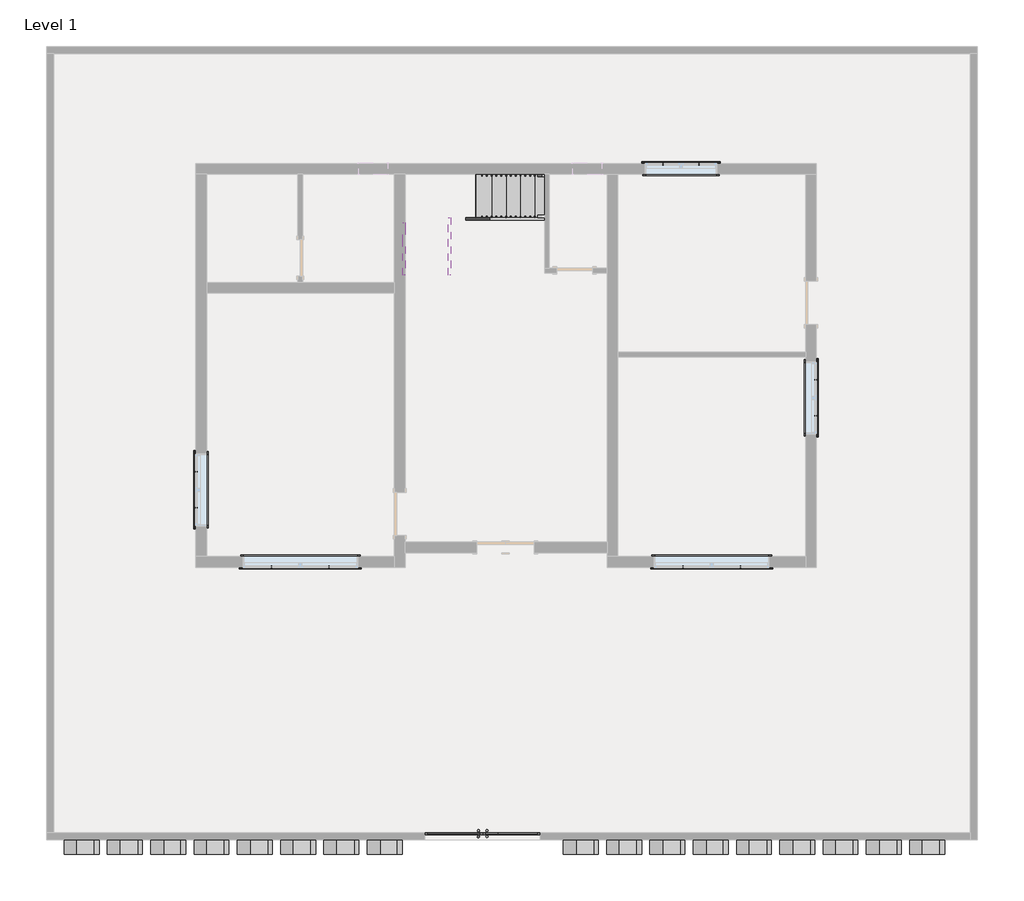
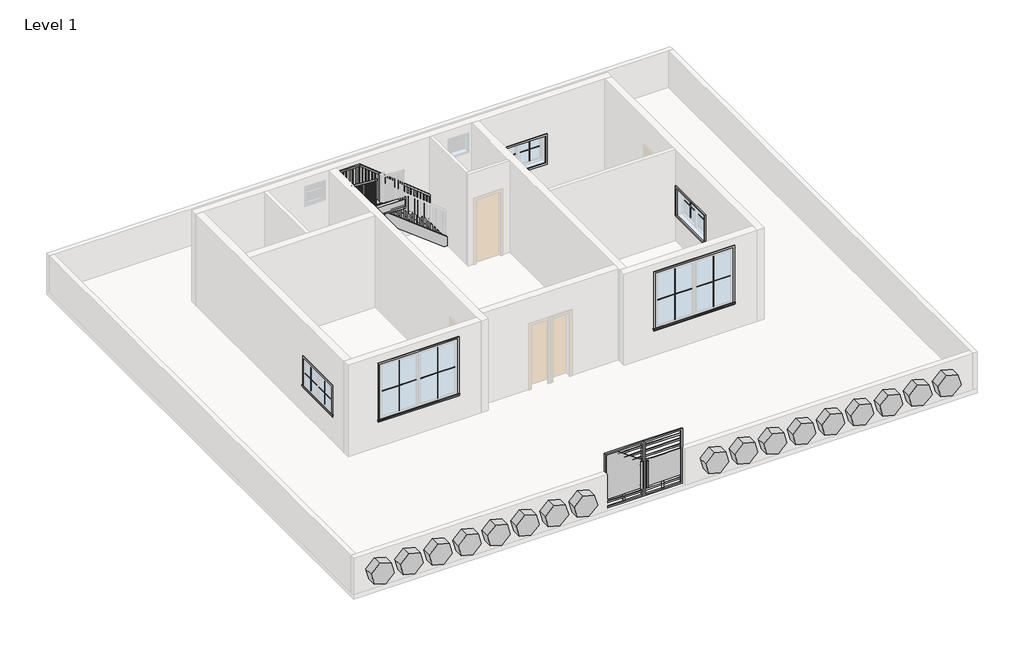
# One storey, part 2 of 2: 38 proxies, 4 members, 1 railing, 1 stair flight.
"""IFC4 building model written with IfcOpenShell, lengths in millimetres."""

from ifc_helpers import new_model, si_unit, frame, origin, place, context, project, spatial, polyline, outline, extrude, faceted_brep, transform, mapped, element, save
from components import generic_models_113f6068, generic_models_1_generic_models_1_e32cbfde, generic_models_10_generic_models_1_db47fcfa, generic_models_11_generic_models_1_4c9ee5e0, generic_models_12_generic_models_1_cd0b2d88, generic_models_13_generic_models_1_344792cf, generic_models_14_generic_models_1_1a1bfa67, generic_models_15_generic_models_1_a1369ee7, generic_models_16_generic_models_1_a0735545, generic_models_17_generic_models_1_fcac293f, generic_models_2_generic_models_1_372cb617, generic_models_3_generic_models_1_c8895c90, generic_models_4_generic_models_1_1de10410, generic_models_5_generic_models_1_6e22be36, generic_models_6_generic_models_1_19455b19, generic_models_7_generic_models_1_35c4f0a6, generic_models_8_generic_models_1_b8e4b7b0, generic_models_9_generic_models_1_cc0d601c, muntin_pattern_2x2_muntin_pattern_2x2_9352d081, muntin_pattern_2x2_muntin_pattern_2x2_5c2cbe28, muntin_pattern_2x2_muntin_pattern_2x2_bb8d4d84, muntin_pattern_2x2_muntin_pattern_2x2_d03a1f3c, trim_window_exterior_flat_with_sill_979bde60, trim_window_exterior_flat_with_sill_359ed2ce, trim_window_interior_flat_picture_frame_7883d11b, trim_window_interior_flat_picture_frame_939a8053, stair_flight_e32d701a

model = new_model("IFC4")

# Units and contexts
model_context = context("Model", 3, world=origin())
ifc_project = project(units=[si_unit("LENGTHUNIT", "METRE", prefix="MILLI")], contexts=[model_context])

# Site, building, storey
site = spatial("IfcSite", under=ifc_project)
building = spatial("IfcBuilding", under=site)
storey = spatial("IfcBuildingStorey", under=building, Name="Level 1", Elevation=0.0)

# Proxies
placement = place(None, origin())
generic_models_shape = generic_models_113f6068(model_context)
element("IfcBuildingElementProxy", 1, Name="Generic Models", at=placement, inside=storey, context=model_context, shape_type="MappedRepresentation", body=[
    mapped(generic_models_shape, transform((-1750.5415084, -8629.4225464, 0.0), x_axis=(1.0, 0.0, 0.0), y_axis=(0.0, 1.0, 0.0), z_axis=(0.0, 0.0, 1.0))),
])
generic_models_1_generic_models_1_shape = generic_models_1_generic_models_1_e32cbfde(model_context)
element("IfcBuildingElementProxy", 2, Name="Generic Models 1 : Generic Models 1", ObjectType="Generic Models 1 : Generic Models 1", at=placement, inside=storey, context=model_context, shape_type="MappedRepresentation", body=[
    mapped(generic_models_1_generic_models_1_shape, transform((0.0, 0.0, 0.0), x_axis=(1.0, 0.0, 0.0), y_axis=(0.0, 1.0, 0.0), z_axis=(0.0, 0.0, 1.0))),
])
generic_models_10_generic_models_1_shape = generic_models_10_generic_models_1_db47fcfa(model_context)
element("IfcBuildingElementProxy", 3, Name="Generic Models 10 : Generic Models 1", ObjectType="Generic Models 10 : Generic Models 1", at=placement, inside=storey, context=model_context, shape_type="MappedRepresentation", body=[
    mapped(generic_models_10_generic_models_1_shape, transform((0.0, 0.0, 0.0), x_axis=(1.0, 0.0, 0.0), y_axis=(0.0, 1.0, 0.0), z_axis=(0.0, 0.0, 1.0))),
])
generic_models_11_generic_models_1_shape = generic_models_11_generic_models_1_4c9ee5e0(model_context)
element("IfcBuildingElementProxy", 4, Name="Generic Models 11 : Generic Models 1", ObjectType="Generic Models 11 : Generic Models 1", at=placement, inside=storey, context=model_context, shape_type="MappedRepresentation", body=[
    mapped(generic_models_11_generic_models_1_shape, transform((0.0, 0.0, 0.0), x_axis=(1.0, 0.0, 0.0), y_axis=(0.0, 1.0, 0.0), z_axis=(0.0, 0.0, 1.0))),
])
generic_models_12_generic_models_1_shape = generic_models_12_generic_models_1_cd0b2d88(model_context)
element("IfcBuildingElementProxy", 5, Name="Generic Models 12 : Generic Models 1", ObjectType="Generic Models 12 : Generic Models 1", at=placement, inside=storey, context=model_context, shape_type="MappedRepresentation", body=[
    mapped(generic_models_12_generic_models_1_shape, transform((0.0, 0.0, 0.0), x_axis=(1.0, 0.0, 0.0), y_axis=(0.0, 1.0, 0.0), z_axis=(0.0, 0.0, 1.0))),
])
generic_models_13_generic_models_1_shape = generic_models_13_generic_models_1_344792cf(model_context)
element("IfcBuildingElementProxy", 6, Name="Generic Models 13 : Generic Models 1", ObjectType="Generic Models 13 : Generic Models 1", at=placement, inside=storey, context=model_context, shape_type="MappedRepresentation", body=[
    mapped(generic_models_13_generic_models_1_shape, transform((0.0, 0.0, 0.0), x_axis=(1.0, 0.0, 0.0), y_axis=(0.0, 1.0, 0.0), z_axis=(0.0, 0.0, 1.0))),
])
generic_models_14_generic_models_1_shape = generic_models_14_generic_models_1_1a1bfa67(model_context)
element("IfcBuildingElementProxy", 7, Name="Generic Models 14 : Generic Models 1", ObjectType="Generic Models 14 : Generic Models 1", at=placement, inside=storey, context=model_context, shape_type="MappedRepresentation", body=[
    mapped(generic_models_14_generic_models_1_shape, transform((0.0, 0.0, 0.0), x_axis=(1.0, 0.0, 0.0), y_axis=(0.0, 1.0, 0.0), z_axis=(0.0, 0.0, 1.0))),
])
generic_models_15_generic_models_1_shape = generic_models_15_generic_models_1_a1369ee7(model_context)
element("IfcBuildingElementProxy", 8, Name="Generic Models 15 : Generic Models 1", ObjectType="Generic Models 15 : Generic Models 1", at=placement, inside=storey, context=model_context, shape_type="MappedRepresentation", body=[
    mapped(generic_models_15_generic_models_1_shape, transform((0.0, 0.0, 0.0), x_axis=(1.0, 0.0, 0.0), y_axis=(0.0, 1.0, 0.0), z_axis=(0.0, 0.0, 1.0))),
])
generic_models_16_generic_models_1_shape = generic_models_16_generic_models_1_a0735545(model_context)
element("IfcBuildingElementProxy", 9, Name="Generic Models 16 : Generic Models 1", ObjectType="Generic Models 16 : Generic Models 1", at=placement, inside=storey, context=model_context, shape_type="MappedRepresentation", body=[
    mapped(generic_models_16_generic_models_1_shape, transform((0.0, 0.0, 0.0), x_axis=(1.0, 0.0, 0.0), y_axis=(0.0, 1.0, 0.0), z_axis=(0.0, 0.0, 1.0))),
])
generic_models_17_generic_models_1_shape = generic_models_17_generic_models_1_fcac293f(model_context)
element("IfcBuildingElementProxy", 10, Name="Generic Models 17 : Generic Models 1", ObjectType="Generic Models 17 : Generic Models 1", at=placement, inside=storey, context=model_context, shape_type="MappedRepresentation", body=[
    mapped(generic_models_17_generic_models_1_shape, transform((0.0, 0.0, 0.0), x_axis=(1.0, 0.0, 0.0), y_axis=(0.0, 1.0, 0.0), z_axis=(0.0, 0.0, 1.0))),
])
generic_models_2_generic_models_1_shape = generic_models_2_generic_models_1_372cb617(model_context)
element("IfcBuildingElementProxy", 11, Name="Generic Models 2 : Generic Models 1", ObjectType="Generic Models 2 : Generic Models 1", at=placement, inside=storey, context=model_context, shape_type="MappedRepresentation", body=[
    mapped(generic_models_2_generic_models_1_shape, transform((0.0, 0.0, 0.0), x_axis=(1.0, 0.0, 0.0), y_axis=(0.0, 1.0, 0.0), z_axis=(0.0, 0.0, 1.0))),
])
generic_models_3_generic_models_1_shape = generic_models_3_generic_models_1_c8895c90(model_context)
element("IfcBuildingElementProxy", 12, Name="Generic Models 3 : Generic Models 1", ObjectType="Generic Models 3 : Generic Models 1", at=placement, inside=storey, context=model_context, shape_type="MappedRepresentation", body=[
    mapped(generic_models_3_generic_models_1_shape, transform((0.0, 0.0, 0.0), x_axis=(1.0, 0.0, 0.0), y_axis=(0.0, 1.0, 0.0), z_axis=(0.0, 0.0, 1.0))),
])
generic_models_4_generic_models_1_shape = generic_models_4_generic_models_1_1de10410(model_context)
element("IfcBuildingElementProxy", 13, Name="Generic Models 4 : Generic Models 1", ObjectType="Generic Models 4 : Generic Models 1", at=placement, inside=storey, context=model_context, shape_type="MappedRepresentation", body=[
    mapped(generic_models_4_generic_models_1_shape, transform((0.0, 0.0, 0.0), x_axis=(1.0, 0.0, 0.0), y_axis=(0.0, 1.0, 0.0), z_axis=(0.0, 0.0, 1.0))),
])
generic_models_5_generic_models_1_shape = generic_models_5_generic_models_1_6e22be36(model_context)
element("IfcBuildingElementProxy", 14, Name="Generic Models 5 : Generic Models 1", ObjectType="Generic Models 5 : Generic Models 1", at=placement, inside=storey, context=model_context, shape_type="MappedRepresentation", body=[
    mapped(generic_models_5_generic_models_1_shape, transform((0.0, 0.0, 0.0), x_axis=(1.0, 0.0, 0.0), y_axis=(0.0, 1.0, 0.0), z_axis=(0.0, 0.0, 1.0))),
])
generic_models_6_generic_models_1_shape = generic_models_6_generic_models_1_19455b19(model_context)
element("IfcBuildingElementProxy", 15, Name="Generic Models 6 : Generic Models 1", ObjectType="Generic Models 6 : Generic Models 1", at=placement, inside=storey, context=model_context, shape_type="MappedRepresentation", body=[
    mapped(generic_models_6_generic_models_1_shape, transform((0.0, 0.0, 0.0), x_axis=(1.0, 0.0, 0.0), y_axis=(0.0, 1.0, 0.0), z_axis=(0.0, 0.0, 1.0))),
])
generic_models_7_generic_models_1_shape = generic_models_7_generic_models_1_35c4f0a6(model_context)
element("IfcBuildingElementProxy", 16, Name="Generic Models 7 : Generic Models 1", ObjectType="Generic Models 7 : Generic Models 1", at=placement, inside=storey, context=model_context, shape_type="MappedRepresentation", body=[
    mapped(generic_models_7_generic_models_1_shape, transform((0.0, 0.0, 0.0), x_axis=(1.0, 0.0, 0.0), y_axis=(0.0, 1.0, 0.0), z_axis=(0.0, 0.0, 1.0))),
])
generic_models_8_generic_models_1_shape = generic_models_8_generic_models_1_b8e4b7b0(model_context)
element("IfcBuildingElementProxy", 17, Name="Generic Models 8 : Generic Models 1", ObjectType="Generic Models 8 : Generic Models 1", at=placement, inside=storey, context=model_context, shape_type="MappedRepresentation", body=[
    mapped(generic_models_8_generic_models_1_shape, transform((0.0, 0.0, 0.0), x_axis=(1.0, 0.0, 0.0), y_axis=(0.0, 1.0, 0.0), z_axis=(0.0, 0.0, 1.0))),
])
generic_models_9_generic_models_1_shape = generic_models_9_generic_models_1_cc0d601c(model_context)
element("IfcBuildingElementProxy", 18, Name="Generic Models 9 : Generic Models 1", ObjectType="Generic Models 9 : Generic Models 1", at=placement, inside=storey, context=model_context, shape_type="MappedRepresentation", body=[
    mapped(generic_models_9_generic_models_1_shape, transform((0.0, 0.0, 0.0), x_axis=(1.0, 0.0, 0.0), y_axis=(0.0, 1.0, 0.0), z_axis=(0.0, 0.0, 1.0))),
])
muntin_pattern_2x2_muntin_pattern_2x2_shape = muntin_pattern_2x2_muntin_pattern_2x2_9352d081(model_context)
element("IfcBuildingElementProxy", 19, Name="Muntin Pattern_2x2 : Muntin Pattern_2x2", ObjectType="Muntin Pattern_2x2 : Muntin Pattern_2x2", at=placement, inside=storey, context=model_context, shape_type="MappedRepresentation", body=[
    mapped(muntin_pattern_2x2_muntin_pattern_2x2_shape, transform((-7798.9165084, -1764.5743005, 984.25), x_axis=(0.0, 1.0, 0.0), y_axis=(-1.0, 0.0, 0.0), z_axis=(0.0, 0.0, 1.0))),
])
element("IfcBuildingElementProxy", 20, Name="Muntin Pattern_2x2 : Muntin Pattern_2x2", ObjectType="Muntin Pattern_2x2 : Muntin Pattern_2x2", at=placement, inside=storey, context=model_context, shape_type="MappedRepresentation", body=[
    mapped(muntin_pattern_2x2_muntin_pattern_2x2_shape, transform((5288.4334916, 937.3506995, 984.25), x_axis=(0.0, -1.0, 0.0), y_axis=(1.0, 0.0, 0.0), z_axis=(0.0, 0.0, 1.0))),
])
element("IfcBuildingElementProxy", 21, Name="Muntin Pattern_2x2 : Muntin Pattern_2x2", ObjectType="Muntin Pattern_2x2 : Muntin Pattern_2x2", at=placement, inside=storey, context=model_context, shape_type="MappedRepresentation", body=[
    mapped(muntin_pattern_2x2_muntin_pattern_2x2_shape, transform((2061.0459916, 5501.4131995, 984.25), x_axis=(1.0, 0.0, 0.0), y_axis=(0.0, 1.0, 0.0), z_axis=(0.0, 0.0, 1.0))),
])
muntin_pattern_2x2_muntin_pattern_2x2_2_shape = muntin_pattern_2x2_muntin_pattern_2x2_5c2cbe28(model_context)
element("IfcBuildingElementProxy", 22, Name="Muntin Pattern_2x2 : Muntin Pattern_2x2", ObjectType="Muntin Pattern_2x2 : Muntin Pattern_2x2", at=placement, inside=storey, context=model_context, shape_type="MappedRepresentation", body=[
    mapped(muntin_pattern_2x2_muntin_pattern_2x2_2_shape, transform((-7798.9165084, -1005.7493005, 984.25), x_axis=(0.0, -1.0, 0.0), y_axis=(1.0, 0.0, 0.0), z_axis=(0.0, 0.0, 1.0))),
])
element("IfcBuildingElementProxy", 23, Name="Muntin Pattern_2x2 : Muntin Pattern_2x2", ObjectType="Muntin Pattern_2x2 : Muntin Pattern_2x2", at=placement, inside=storey, context=model_context, shape_type="MappedRepresentation", body=[
    mapped(muntin_pattern_2x2_muntin_pattern_2x2_2_shape, transform((5288.4334916, 178.5256995, 984.25), x_axis=(0.0, 1.0, 0.0), y_axis=(-1.0, 0.0, 0.0), z_axis=(0.0, 0.0, 1.0))),
])
element("IfcBuildingElementProxy", 24, Name="Muntin Pattern_2x2 : Muntin Pattern_2x2", ObjectType="Muntin Pattern_2x2 : Muntin Pattern_2x2", at=placement, inside=storey, context=model_context, shape_type="MappedRepresentation", body=[
    mapped(muntin_pattern_2x2_muntin_pattern_2x2_2_shape, transform((2819.8709916, 5501.4131995, 984.25), x_axis=(-1.0, 0.0, 0.0), y_axis=(0.0, -1.0, 0.0), z_axis=(0.0, 0.0, 1.0))),
])
muntin_pattern_2x2_muntin_pattern_2x2_3_shape = muntin_pattern_2x2_muntin_pattern_2x2_bb8d4d84(model_context)
element("IfcBuildingElementProxy", 25, Name="Muntin Pattern_2x2 : Muntin Pattern_2x2", ObjectType="Muntin Pattern_2x2 : Muntin Pattern_2x2", at=placement, inside=storey, context=model_context, shape_type="MappedRepresentation", body=[
    mapped(muntin_pattern_2x2_muntin_pattern_2x2_3_shape, transform((-4990.6290084, -3013.9368005, 984.25), x_axis=(-1.0, 0.0, 0.0), y_axis=(0.0, -1.0, 0.0), z_axis=(0.0, 0.0, 1.0))),
])
element("IfcBuildingElementProxy", 26, Name="Muntin Pattern_2x2 : Muntin Pattern_2x2", ObjectType="Muntin Pattern_2x2 : Muntin Pattern_2x2", at=placement, inside=storey, context=model_context, shape_type="MappedRepresentation", body=[
    mapped(muntin_pattern_2x2_muntin_pattern_2x2_3_shape, transform((3696.1709916, -3013.9368005, 984.25), x_axis=(-1.0, 0.0, 0.0), y_axis=(0.0, -1.0, 0.0), z_axis=(0.0, 0.0, 1.0))),
])
muntin_pattern_2x2_muntin_pattern_2x2_4_shape = muntin_pattern_2x2_muntin_pattern_2x2_d03a1f3c(model_context)
element("IfcBuildingElementProxy", 27, Name="Muntin Pattern_2x2 : Muntin Pattern_2x2", ObjectType="Muntin Pattern_2x2 : Muntin Pattern_2x2", at=placement, inside=storey, context=model_context, shape_type="MappedRepresentation", body=[
    mapped(muntin_pattern_2x2_muntin_pattern_2x2_4_shape, transform((-6206.6540084, -3013.9368005, 984.25), x_axis=(1.0, 0.0, 0.0), y_axis=(0.0, 1.0, 0.0), z_axis=(0.0, 0.0, 1.0))),
])
element("IfcBuildingElementProxy", 28, Name="Muntin Pattern_2x2 : Muntin Pattern_2x2", ObjectType="Muntin Pattern_2x2 : Muntin Pattern_2x2", at=placement, inside=storey, context=model_context, shape_type="MappedRepresentation", body=[
    mapped(muntin_pattern_2x2_muntin_pattern_2x2_4_shape, transform((2480.1459916, -3013.9368005, 984.25), x_axis=(1.0, 0.0, 0.0), y_axis=(0.0, 1.0, 0.0), z_axis=(0.0, 0.0, 1.0))),
])
trim_window_exterior_flat_with_sill_shape = trim_window_exterior_flat_with_sill_979bde60(model_context)
element("IfcBuildingElementProxy", 29, Name="Trim-Window-Exterior-Flat : with Sill", ObjectType="Trim-Window-Exterior-Flat : with Sill", at=placement, inside=storey, context=model_context, shape_type="MappedRepresentation", body=[
    mapped(trim_window_exterior_flat_with_sill_shape, transform((-7808.4415084, -1385.1618005, 1828.8), x_axis=(0.0, -1.0, 0.0), y_axis=(0.0, 0.0, 1.0), z_axis=(-1.0, 0.0, 0.0))),
])
element("IfcBuildingElementProxy", 30, Name="Trim-Window-Exterior-Flat : with Sill", ObjectType="Trim-Window-Exterior-Flat : with Sill", at=placement, inside=storey, context=model_context, shape_type="MappedRepresentation", body=[
    mapped(trim_window_exterior_flat_with_sill_shape, transform((5297.9584916, 557.9381995, 1828.8), x_axis=(0.0, 1.0, 0.0), y_axis=(0.0, 0.0, 1.0), z_axis=(1.0, 0.0, 0.0))),
])
element("IfcBuildingElementProxy", 31, Name="Trim-Window-Exterior-Flat : with Sill", ObjectType="Trim-Window-Exterior-Flat : with Sill", at=placement, inside=storey, context=model_context, shape_type="MappedRepresentation", body=[
    mapped(trim_window_exterior_flat_with_sill_shape, transform((2440.4584916, 5510.9381995, 1828.8), x_axis=(-1.0, 0.0, 0.0), y_axis=(0.0, 0.0, 1.0), z_axis=(0.0, 1.0, 0.0))),
])
trim_window_exterior_flat_with_sill_2_shape = trim_window_exterior_flat_with_sill_359ed2ce(model_context)
element("IfcBuildingElementProxy", 32, Name="Trim-Window-Exterior-Flat : with Sill", ObjectType="Trim-Window-Exterior-Flat : with Sill", at=placement, inside=storey, context=model_context, shape_type="MappedRepresentation", body=[
    mapped(trim_window_exterior_flat_with_sill_2_shape, transform((-5598.6415084, -3023.4618005, 2743.2), x_axis=(1.0, 0.0, 0.0), y_axis=(0.0, 0.0, 1.0), z_axis=(0.0, -1.0, 0.0))),
])
element("IfcBuildingElementProxy", 33, Name="Trim-Window-Exterior-Flat : with Sill", ObjectType="Trim-Window-Exterior-Flat : with Sill", at=placement, inside=storey, context=model_context, shape_type="MappedRepresentation", body=[
    mapped(trim_window_exterior_flat_with_sill_2_shape, transform((3088.1584916, -3023.4618005, 2743.2), x_axis=(1.0, 0.0, 0.0), y_axis=(0.0, 0.0, 1.0), z_axis=(0.0, -1.0, 0.0))),
])
trim_window_interior_flat_picture_frame_shape = trim_window_interior_flat_picture_frame_7883d11b(model_context)
element("IfcBuildingElementProxy", 34, Name="Trim-Window-Interior-Flat : Picture Frame", ObjectType="Trim-Window-Interior-Flat : Picture Frame", at=placement, inside=storey, context=model_context, shape_type="MappedRepresentation", body=[
    mapped(trim_window_interior_flat_picture_frame_shape, transform((-7579.8415084, -1385.1618005, 1828.8), x_axis=(0.0, 1.0, 0.0), y_axis=(0.0, 0.0, 1.0), z_axis=(1.0, 0.0, 0.0))),
])
element("IfcBuildingElementProxy", 35, Name="Trim-Window-Interior-Flat : Picture Frame", ObjectType="Trim-Window-Interior-Flat : Picture Frame", at=placement, inside=storey, context=model_context, shape_type="MappedRepresentation", body=[
    mapped(trim_window_interior_flat_picture_frame_shape, transform((5069.3584916, 557.9381995, 1828.8), x_axis=(0.0, -1.0, 0.0), y_axis=(0.0, 0.0, 1.0), z_axis=(-1.0, 0.0, 0.0))),
])
element("IfcBuildingElementProxy", 36, Name="Trim-Window-Interior-Flat : Picture Frame", ObjectType="Trim-Window-Interior-Flat : Picture Frame", at=placement, inside=storey, context=model_context, shape_type="MappedRepresentation", body=[
    mapped(trim_window_interior_flat_picture_frame_shape, transform((2440.4584916, 5282.3381995, 1828.8), x_axis=(1.0, 0.0, 0.0), y_axis=(0.0, 0.0, 1.0), z_axis=(0.0, -1.0, 0.0))),
])
trim_window_interior_flat_picture_frame_2_shape = trim_window_interior_flat_picture_frame_939a8053(model_context)
element("IfcBuildingElementProxy", 37, Name="Trim-Window-Interior-Flat : Picture Frame", ObjectType="Trim-Window-Interior-Flat : Picture Frame", at=placement, inside=storey, context=model_context, shape_type="MappedRepresentation", body=[
    mapped(trim_window_interior_flat_picture_frame_2_shape, transform((-5598.6415084, -2794.8618005, 2743.2), x_axis=(-1.0, 0.0, 0.0), y_axis=(0.0, 0.0, 1.0), z_axis=(0.0, 1.0, 0.0))),
])
element("IfcBuildingElementProxy", 38, Name="Trim-Window-Interior-Flat : Picture Frame", ObjectType="Trim-Window-Interior-Flat : Picture Frame", at=placement, inside=storey, context=model_context, shape_type="MappedRepresentation", body=[
    mapped(trim_window_interior_flat_picture_frame_2_shape, transform((3088.1584916, -2794.8618005, 2743.2), x_axis=(-1.0, 0.0, 0.0), y_axis=(0.0, 0.0, 1.0), z_axis=(0.0, 1.0, 0.0))),
])

# Members
element("IfcMember", 39, ObjectType="Stringer - 2\" Width", at=placement, inside=storey, context=model_context, shape_type="SweptSolid", body=[
    extrude(outline(polyline([(0.0, -442.4415084), (307.3626352, -442.4415084), (1831.3626352, -2423.6415084), (1446.8171203, -2423.6415084), (0.0, -542.779252), (0.0, -442.4415084)])), frame((0.0, 4317.5146777, 0.0), z_axis=(0.0, 1.0, 0.0), x_axis=(0.0, 0.0, 1.0)), (0.0, 0.0, 1.0), 50.8),
])
element("IfcMember", 40, ObjectType="Stringer - 2\" Width", at=placement, inside=storey, context=model_context, shape_type="SweptSolid", body=[
    extrude(outline(polyline([(4368.3146777, 2104.8645881), (4368.3146777, 1720.3778824), (3148.7383287, 2658.1275497), (3148.7383287, 3042.6142554), (4368.3146777, 2104.8645881)])), frame((-2474.4415084, 0.0, 0.0), z_axis=(1.0, 0.0, 0.0), x_axis=(0.0, 1.0, 0.0)), (0.0, 0.0, 1.0), 50.8),
])
element("IfcMember", 41, ObjectType="Stringer - 2\" Width", at=placement, inside=storey, context=model_context, shape_type="SweptSolid", body=[
    extrude(outline(polyline([(0.0, -442.4415084), (307.3626352, -442.4415084), (1402.0588522, -1865.5465904), (1402.0588522, -2365.4557598), (0.0, -542.779252), (0.0, -442.4415084)])), frame((0.0, 5282.3381995, 0.0), z_axis=(0.0, 1.0, 0.0), x_axis=(0.0, 0.0, 1.0)), (0.0, 0.0, 1.0), 50.8),
])
element("IfcMember", 42, ObjectType="Stringer - 2\" Width", at=placement, inside=storey, context=model_context, shape_type="SweptSolid", body=[
    extrude(outline(polyline([(3758.4927637, 2189.2786588), (3148.7383287, 2658.1275497), (3148.7383287, 3042.6142554), (4258.5312166, 2189.2786588), (3758.4927637, 2189.2786588)])), frame((-3439.6415084, 0.0, 0.0), z_axis=(1.0, 0.0, 0.0), x_axis=(0.0, 1.0, 0.0)), (0.0, 0.0, 1.0), 50.8),
])

# Railing
element("IfcRailing", 43, ObjectType="Handrail - Rectangular", at=placement, inside=storey, context=model_context, shape_type="SolidModel", body=[
    faceted_brep([(-442.4415084, 5231.5381995, 1148.8615385), (-442.4415084, 5231.5381995, 1083.5609717), (-442.4415084, 5282.3381995, 1083.5609717), (-442.4415084, 5282.3381995, 1148.8615385), (-2641.0608886, 5231.5381995, 2924.6694994), (-2659.0139713, 5231.5381995, 2873.8694994), (-2659.0139713, 5282.3381995, 2873.8694994), (-2641.0608886, 5282.3381995, 2924.6694994), (-3338.0415084, 5231.5381995, 2924.6694994), (-3338.0415084, 5231.5381995, 2873.8694994), (-3388.8415084, 5282.3381995, 2873.8694994), (-3388.8415084, 5282.3381995, 2924.6694994), (-3338.0415084, 4498.2044111, 2924.6694994), (-3338.0415084, 4480.9304428, 2873.8694994), (-3388.8415084, 4480.9304428, 2873.8694994), (-3388.8415084, 4498.2044111, 2924.6694994), (-3338.0415084, 3148.7383287, 3962.4), (-3388.8415084, 3148.7383287, 3962.4), (-3388.8415084, 3148.7383287, 3898.3164325), (-3338.0415084, 3148.7383287, 3898.3164325)], [[[0, 1, 2, 3]], [[1, 0, 4, 5]], [[2, 1, 5, 6]], [[3, 2, 6, 7]], [[0, 3, 7, 4]], [[5, 4, 8, 9]], [[6, 5, 9, 10]], [[7, 6, 10, 11]], [[4, 7, 11, 8]], [[9, 8, 12, 13]], [[10, 9, 13, 14]], [[11, 10, 14, 15]], [[8, 11, 15, 12]], [[16, 17, 18, 19]], [[13, 12, 16, 19]], [[14, 13, 19, 18]], [[15, 14, 18, 17]], [[12, 15, 17, 16]]]),
    extrude(outline(polyline([(3215.4131995, 3847.1162499), (3234.4631995, 3832.4669257), (3234.4631995, 2813.5384615), (3215.4131995, 2813.5384615), (3215.4131995, 3847.1162499)])), frame((-3372.9665084, 0.0, 0.0), z_axis=(1.0, 0.0, 0.0), x_axis=(0.0, 1.0, 0.0)), (0.0, 0.0, 1.0), 19.05),
    extrude(outline(polyline([(3317.0131995, 3768.9141687), (3336.0631995, 3754.2648446), (3336.0631995, 2813.5384615), (3317.0131995, 2813.5384615), (3317.0131995, 3768.9141687)])), frame((-3372.9665084, 0.0, 0.0), z_axis=(1.0, 0.0, 0.0), x_axis=(0.0, 1.0, 0.0)), (0.0, 0.0, 1.0), 19.05),
    extrude(outline(polyline([(3418.6131995, 3690.7844401), (3437.6631995, 3676.1351159), (3437.6631995, 2813.5384615), (3418.6131995, 2813.5384615), (3418.6131995, 3690.7844401)])), frame((-3372.9665084, 0.0, 0.0), z_axis=(1.0, 0.0, 0.0), x_axis=(0.0, 1.0, 0.0)), (0.0, 0.0, 1.0), 19.05),
    extrude(outline(polyline([(3520.2131995, 3612.6547114), (3539.2631995, 3598.0053873), (3539.2631995, 2579.0769231), (3520.2131995, 2579.0769231), (3520.2131995, 3612.6547114)])), frame((-3372.9665084, 0.0, 0.0), z_axis=(1.0, 0.0, 0.0), x_axis=(0.0, 1.0, 0.0)), (0.0, 0.0, 1.0), 19.05),
    extrude(outline(polyline([(3621.8131995, 3534.6696877), (3640.8631995, 3520.0203636), (3640.8631995, 2579.0769231), (3621.8131995, 2579.0769231), (3621.8131995, 3534.6696877)])), frame((-3372.9665084, 0.0, 0.0), z_axis=(1.0, 0.0, 0.0), x_axis=(0.0, 1.0, 0.0)), (0.0, 0.0, 1.0), 19.05),
    extrude(outline(polyline([(3723.4131995, 3456.539959), (3742.4631995, 3441.8906349), (3742.4631995, 2579.0769231), (3723.4131995, 2579.0769231), (3723.4131995, 3456.539959)])), frame((-3372.9665084, 0.0, 0.0), z_axis=(1.0, 0.0, 0.0), x_axis=(0.0, 1.0, 0.0)), (0.0, 0.0, 1.0), 19.05),
    extrude(outline(polyline([(3825.0131995, 3378.4102304), (3844.0631995, 3363.7609063), (3844.0631995, 2344.6153846), (3825.0131995, 2344.6153846), (3825.0131995, 3378.4102304)])), frame((-3372.9665084, 0.0, 0.0), z_axis=(1.0, 0.0, 0.0), x_axis=(0.0, 1.0, 0.0)), (0.0, 0.0, 1.0), 19.05),
    extrude(outline(polyline([(3926.6131995, 3300.2081492), (3945.6631995, 3285.5588251), (3945.6631995, 2344.6153846), (3926.6131995, 2344.6153846), (3926.6131995, 3300.2081492)])), frame((-3372.9665084, 0.0, 0.0), z_axis=(1.0, 0.0, 0.0), x_axis=(0.0, 1.0, 0.0)), (0.0, 0.0, 1.0), 19.05),
    extrude(outline(polyline([(4028.2131995, 3222.0784206), (4047.2631995, 3207.4290965), (4047.2631995, 2344.6153846), (4028.2131995, 2344.6153846), (4028.2131995, 3222.0784206)])), frame((-3372.9665084, 0.0, 0.0), z_axis=(1.0, 0.0, 0.0), x_axis=(0.0, 1.0, 0.0)), (0.0, 0.0, 1.0), 19.05),
    extrude(outline(polyline([(4129.8131995, 3143.9486919), (4148.8631995, 3129.2993678), (4148.8631995, 2110.1538462), (4129.8131995, 2110.1538462), (4129.8131995, 3143.9486919)])), frame((-3372.9665084, 0.0, 0.0), z_axis=(1.0, 0.0, 0.0), x_axis=(0.0, 1.0, 0.0)), (0.0, 0.0, 1.0), 19.05),
    extrude(outline(polyline([(4231.4131995, 3065.7466108), (4250.4631995, 3051.0972867), (4250.4631995, 2110.1538462), (4231.4131995, 2110.1538462), (4231.4131995, 3065.7466108)])), frame((-3372.9665084, 0.0, 0.0), z_axis=(1.0, 0.0, 0.0), x_axis=(0.0, 1.0, 0.0)), (0.0, 0.0, 1.0), 19.05),
    extrude(outline(polyline([(4333.0131995, 2987.6168821), (4352.0631995, 2972.967558), (4352.0631995, 2110.1538462), (4333.0131995, 2110.1538462), (4333.0131995, 2987.6168821)])), frame((-3372.9665084, 0.0, 0.0), z_axis=(1.0, 0.0, 0.0), x_axis=(0.0, 1.0, 0.0)), (0.0, 0.0, 1.0), 19.05),
    extrude(outline(polyline([(4434.6131995, 2909.4871535), (4453.6631995, 2894.8378293), (4453.6631995, 1875.6923077), (4434.6131995, 1875.6923077), (4434.6131995, 2909.4871535)])), frame((-3372.9665084, 0.0, 0.0), z_axis=(1.0, 0.0, 0.0), x_axis=(0.0, 1.0, 0.0)), (0.0, 0.0, 1.0), 19.05),
    extrude(outline(polyline([(-3372.9665084, 4555.2631995), (-3353.9165084, 4555.2631995), (-3353.9165084, 4536.2131995), (-3372.9665084, 4536.2131995), (-3372.9665084, 4555.2631995)])), frame((0.0, 0.0, 1875.6923077), z_axis=(0.0, 0.0, 1.0), x_axis=(1.0, 0.0, 0.0)), (0.0, 0.0, 1.0), 998.1771917),
    extrude(outline(polyline([(-3372.9665084, 4656.8631995), (-3353.9165084, 4656.8631995), (-3353.9165084, 4637.8131995), (-3372.9665084, 4637.8131995), (-3372.9665084, 4656.8631995)])), frame((0.0, 0.0, 1875.6923077), z_axis=(0.0, 0.0, 1.0), x_axis=(1.0, 0.0, 0.0)), (0.0, 0.0, 1.0), 998.1771917),
    extrude(outline(polyline([(-3372.9665084, 4758.4631995), (-3353.9165084, 4758.4631995), (-3353.9165084, 4739.4131995), (-3372.9665084, 4739.4131995), (-3372.9665084, 4758.4631995)])), frame((0.0, 0.0, 1875.6923077), z_axis=(0.0, 0.0, 1.0), x_axis=(1.0, 0.0, 0.0)), (0.0, 0.0, 1.0), 998.1771917),
    extrude(outline(polyline([(-3372.9665084, 4860.0631995), (-3353.9165084, 4860.0631995), (-3353.9165084, 4841.0131995), (-3372.9665084, 4841.0131995), (-3372.9665084, 4860.0631995)])), frame((0.0, 0.0, 1875.6923077), z_axis=(0.0, 0.0, 1.0), x_axis=(1.0, 0.0, 0.0)), (0.0, 0.0, 1.0), 998.1771917),
    extrude(outline(polyline([(-3372.9665084, 4961.6631995), (-3353.9165084, 4961.6631995), (-3353.9165084, 4942.6131995), (-3372.9665084, 4942.6131995), (-3372.9665084, 4961.6631995)])), frame((0.0, 0.0, 1875.6923077), z_axis=(0.0, 0.0, 1.0), x_axis=(1.0, 0.0, 0.0)), (0.0, 0.0, 1.0), 998.1771917),
    extrude(outline(polyline([(-3372.9665084, 5063.2631995), (-3353.9165084, 5063.2631995), (-3353.9165084, 5044.2131995), (-3372.9665084, 5044.2131995), (-3372.9665084, 5063.2631995)])), frame((0.0, 0.0, 1875.6923077), z_axis=(0.0, 0.0, 1.0), x_axis=(1.0, 0.0, 0.0)), (0.0, 0.0, 1.0), 998.1771917),
    extrude(outline(polyline([(-3372.9665084, 5164.8631995), (-3353.9165084, 5164.8631995), (-3353.9165084, 5145.8131995), (-3372.9665084, 5145.8131995), (-3372.9665084, 5164.8631995)])), frame((0.0, 0.0, 1875.6923077), z_axis=(0.0, 0.0, 1.0), x_axis=(1.0, 0.0, 0.0)), (0.0, 0.0, 1.0), 998.1771917),
    extrude(outline(polyline([(-3277.7165084, 5266.4631995), (-3277.7165084, 5247.4131995), (-3296.7665084, 5247.4131995), (-3296.7665084, 5266.4631995), (-3277.7165084, 5266.4631995)])), frame((0.0, 0.0, 1875.6923077), z_axis=(0.0, 0.0, 1.0), x_axis=(1.0, 0.0, 0.0)), (0.0, 0.0, 1.0), 998.1771917),
    extrude(outline(polyline([(-3176.1165084, 5266.4631995), (-3176.1165084, 5247.4131995), (-3195.1665084, 5247.4131995), (-3195.1665084, 5266.4631995), (-3176.1165084, 5266.4631995)])), frame((0.0, 0.0, 1875.6923077), z_axis=(0.0, 0.0, 1.0), x_axis=(1.0, 0.0, 0.0)), (0.0, 0.0, 1.0), 998.1771917),
    extrude(outline(polyline([(-3074.5165084, 5266.4631995), (-3074.5165084, 5247.4131995), (-3093.5665084, 5247.4131995), (-3093.5665084, 5266.4631995), (-3074.5165084, 5266.4631995)])), frame((0.0, 0.0, 1875.6923077), z_axis=(0.0, 0.0, 1.0), x_axis=(1.0, 0.0, 0.0)), (0.0, 0.0, 1.0), 998.1771917),
    extrude(outline(polyline([(-2972.9165084, 5266.4631995), (-2972.9165084, 5247.4131995), (-2991.9665084, 5247.4131995), (-2991.9665084, 5266.4631995), (-2972.9165084, 5266.4631995)])), frame((0.0, 0.0, 1875.6923077), z_axis=(0.0, 0.0, 1.0), x_axis=(1.0, 0.0, 0.0)), (0.0, 0.0, 1.0), 998.1771917),
    extrude(outline(polyline([(-2871.3165084, 5266.4631995), (-2871.3165084, 5247.4131995), (-2890.3665084, 5247.4131995), (-2890.3665084, 5266.4631995), (-2871.3165084, 5266.4631995)])), frame((0.0, 0.0, 1875.6923077), z_axis=(0.0, 0.0, 1.0), x_axis=(1.0, 0.0, 0.0)), (0.0, 0.0, 1.0), 998.1771917),
    extrude(outline(polyline([(-2769.7165084, 5266.4631995), (-2769.7165084, 5247.4131995), (-2788.7665084, 5247.4131995), (-2788.7665084, 5266.4631995), (-2769.7165084, 5266.4631995)])), frame((0.0, 0.0, 1875.6923077), z_axis=(0.0, 0.0, 1.0), x_axis=(1.0, 0.0, 0.0)), (0.0, 0.0, 1.0), 998.1771917),
    extrude(outline(polyline([(-2668.1165084, 5266.4631995), (-2668.1165084, 5247.4131995), (-2687.1665084, 5247.4131995), (-2687.1665084, 5266.4631995), (-2668.1165084, 5266.4631995)])), frame((0.0, 0.0, 1875.6923077), z_axis=(0.0, 0.0, 1.0), x_axis=(1.0, 0.0, 0.0)), (0.0, 0.0, 1.0), 998.1771917),
    extrude(outline(polyline([(2799.1600101, -2566.5165084), (2814.5465486, -2585.5665084), (1875.6923077, -2585.5665084), (1875.6923077, -2566.5165084), (2799.1600101, -2566.5165084)])), frame((0.0, 5247.4131995, 0.0), z_axis=(0.0, 1.0, 0.0), x_axis=(0.0, 0.0, 1.0)), (0.0, 0.0, 1.0), 19.05),
    extrude(outline(polyline([(2717.0984717, -2464.9165084), (2732.4850101, -2483.9665084), (1875.6923077, -2483.9665084), (1875.6923077, -2464.9165084), (2717.0984717, -2464.9165084)])), frame((0.0, 5247.4131995, 0.0), z_axis=(0.0, 1.0, 0.0), x_axis=(0.0, 0.0, 1.0)), (0.0, 0.0, 1.0), 19.05),
    extrude(outline(polyline([(2635.0369332, -2363.3165084), (2650.4234717, -2382.3665084), (1641.2307692, -2382.3665084), (1641.2307692, -2363.3165084), (2635.0369332, -2363.3165084)])), frame((0.0, 5247.4131995, 0.0), z_axis=(0.0, 1.0, 0.0), x_axis=(0.0, 0.0, 1.0)), (0.0, 0.0, 1.0), 19.05),
    extrude(outline(polyline([(2552.9753947, -2261.7165084), (2568.3619332, -2280.7665084), (1641.2307692, -2280.7665084), (1641.2307692, -2261.7165084), (2552.9753947, -2261.7165084)])), frame((0.0, 5247.4131995, 0.0), z_axis=(0.0, 1.0, 0.0), x_axis=(0.0, 0.0, 1.0)), (0.0, 0.0, 1.0), 19.05),
    extrude(outline(polyline([(2470.9138563, -2160.1165084), (2486.3003947, -2179.1665084), (1641.2307692, -2179.1665084), (1641.2307692, -2160.1165084), (2470.9138563, -2160.1165084)])), frame((0.0, 5247.4131995, 0.0), z_axis=(0.0, 1.0, 0.0), x_axis=(0.0, 0.0, 1.0)), (0.0, 0.0, 1.0), 19.05),
    extrude(outline(polyline([(2388.8523178, -2058.5165084), (2404.2388563, -2077.5665084), (1406.7692308, -2077.5665084), (1406.7692308, -2058.5165084), (2388.8523178, -2058.5165084)])), frame((0.0, 5247.4131995, 0.0), z_axis=(0.0, 1.0, 0.0), x_axis=(0.0, 0.0, 1.0)), (0.0, 0.0, 1.0), 19.05),
    extrude(outline(polyline([(2306.7907794, -1956.9165084), (2322.1773178, -1975.9665084), (1406.7692308, -1975.9665084), (1406.7692308, -1956.9165084), (2306.7907794, -1956.9165084)])), frame((0.0, 5247.4131995, 0.0), z_axis=(0.0, 1.0, 0.0), x_axis=(0.0, 0.0, 1.0)), (0.0, 0.0, 1.0), 19.05),
    extrude(outline(polyline([(2224.7292409, -1855.3165084), (2240.1157794, -1874.3665084), (1406.7692308, -1874.3665084), (1406.7692308, -1855.3165084), (2224.7292409, -1855.3165084)])), frame((0.0, 5247.4131995, 0.0), z_axis=(0.0, 1.0, 0.0), x_axis=(0.0, 0.0, 1.0)), (0.0, 0.0, 1.0), 19.05),
    extrude(outline(polyline([(2142.6677024, -1753.7165084), (2158.0542409, -1772.7665084), (1172.3076923, -1772.7665084), (1172.3076923, -1753.7165084), (2142.6677024, -1753.7165084)])), frame((0.0, 5247.4131995, 0.0), z_axis=(0.0, 1.0, 0.0), x_axis=(0.0, 0.0, 1.0)), (0.0, 0.0, 1.0), 19.05),
    extrude(outline(polyline([(2060.606164, -1652.1165084), (2075.9927024, -1671.1665084), (1172.3076923, -1671.1665084), (1172.3076923, -1652.1165084), (2060.606164, -1652.1165084)])), frame((0.0, 5247.4131995, 0.0), z_axis=(0.0, 1.0, 0.0), x_axis=(0.0, 0.0, 1.0)), (0.0, 0.0, 1.0), 19.05),
    extrude(outline(polyline([(1978.5446255, -1550.5165084), (1993.931164, -1569.5665084), (1172.3076923, -1569.5665084), (1172.3076923, -1550.5165084), (1978.5446255, -1550.5165084)])), frame((0.0, 5247.4131995, 0.0), z_axis=(0.0, 1.0, 0.0), x_axis=(0.0, 0.0, 1.0)), (0.0, 0.0, 1.0), 19.05),
    extrude(outline(polyline([(1896.4830871, -1448.9165084), (1911.8696255, -1467.9665084), (937.8461538, -1467.9665084), (937.8461538, -1448.9165084), (1896.4830871, -1448.9165084)])), frame((0.0, 5247.4131995, 0.0), z_axis=(0.0, 1.0, 0.0), x_axis=(0.0, 0.0, 1.0)), (0.0, 0.0, 1.0), 19.05),
    extrude(outline(polyline([(1814.4215486, -1347.3165084), (1829.8080871, -1366.3665084), (937.8461538, -1366.3665084), (937.8461538, -1347.3165084), (1814.4215486, -1347.3165084)])), frame((0.0, 5247.4131995, 0.0), z_axis=(0.0, 1.0, 0.0), x_axis=(0.0, 0.0, 1.0)), (0.0, 0.0, 1.0), 19.05),
    extrude(outline(polyline([(1732.3600101, -1245.7165084), (1747.7465486, -1264.7665084), (937.8461538, -1264.7665084), (937.8461538, -1245.7165084), (1732.3600101, -1245.7165084)])), frame((0.0, 5247.4131995, 0.0), z_axis=(0.0, 1.0, 0.0), x_axis=(0.0, 0.0, 1.0)), (0.0, 0.0, 1.0), 19.05),
    extrude(outline(polyline([(1650.2984717, -1144.1165084), (1665.6850101, -1163.1665084), (703.3846154, -1163.1665084), (703.3846154, -1144.1165084), (1650.2984717, -1144.1165084)])), frame((0.0, 5247.4131995, 0.0), z_axis=(0.0, 1.0, 0.0), x_axis=(0.0, 0.0, 1.0)), (0.0, 0.0, 1.0), 19.05),
    extrude(outline(polyline([(1568.2369332, -1042.5165084), (1583.6234717, -1061.5665084), (703.3846154, -1061.5665084), (703.3846154, -1042.5165084), (1568.2369332, -1042.5165084)])), frame((0.0, 5247.4131995, 0.0), z_axis=(0.0, 1.0, 0.0), x_axis=(0.0, 0.0, 1.0)), (0.0, 0.0, 1.0), 19.05),
    extrude(outline(polyline([(1486.1753947, -940.9165084), (1501.5619332, -959.9665084), (703.3846154, -959.9665084), (703.3846154, -940.9165084), (1486.1753947, -940.9165084)])), frame((0.0, 5247.4131995, 0.0), z_axis=(0.0, 1.0, 0.0), x_axis=(0.0, 0.0, 1.0)), (0.0, 0.0, 1.0), 19.05),
    extrude(outline(polyline([(1404.1138563, -839.3165084), (1419.5003947, -858.3665084), (468.9230769, -858.3665084), (468.9230769, -839.3165084), (1404.1138563, -839.3165084)])), frame((0.0, 5247.4131995, 0.0), z_axis=(0.0, 1.0, 0.0), x_axis=(0.0, 0.0, 1.0)), (0.0, 0.0, 1.0), 19.05),
    extrude(outline(polyline([(1322.0523178, -737.7165084), (1337.4388563, -756.7665084), (468.9230769, -756.7665084), (468.9230769, -737.7165084), (1322.0523178, -737.7165084)])), frame((0.0, 5247.4131995, 0.0), z_axis=(0.0, 1.0, 0.0), x_axis=(0.0, 0.0, 1.0)), (0.0, 0.0, 1.0), 19.05),
    extrude(outline(polyline([(1239.9907794, -636.1165084), (1255.3773178, -655.1665084), (468.9230769, -655.1665084), (468.9230769, -636.1165084), (1239.9907794, -636.1165084)])), frame((0.0, 5247.4131995, 0.0), z_axis=(0.0, 1.0, 0.0), x_axis=(0.0, 0.0, 1.0)), (0.0, 0.0, 1.0), 19.05),
    extrude(outline(polyline([(1157.9292409, -534.5165084), (1173.3157794, -553.5665084), (234.4615385, -553.5665084), (234.4615385, -534.5165084), (1157.9292409, -534.5165084)])), frame((0.0, 5247.4131995, 0.0), z_axis=(0.0, 1.0, 0.0), x_axis=(0.0, 0.0, 1.0)), (0.0, 0.0, 1.0), 19.05),
    extrude(outline(polyline([(-3353.9165084, 5266.4631995), (-3353.9165084, 5247.4131995), (-3372.9665084, 5247.4131995), (-3372.9665084, 5266.4631995), (-3353.9165084, 5266.4631995)])), frame((0.0, 0.0, 1875.6923077), z_axis=(0.0, 0.0, 1.0), x_axis=(1.0, 0.0, 0.0)), (0.0, 0.0, 1.0), 998.1771917),
    extrude(outline(polyline([(3148.7383287, 3898.3164325), (3167.7883287, 3883.6671084), (3167.7883287, 2813.5384615), (3148.7383287, 2813.5384615), (3148.7383287, 3898.3164325)])), frame((-3372.9665084, 0.0, 0.0), z_axis=(1.0, 0.0, 0.0), x_axis=(0.0, 1.0, 0.0)), (0.0, 0.0, 1.0), 19.05),
    extrude(outline(polyline([(1083.5609717, -442.4415084), (1098.9475101, -461.4915084), (234.4615385, -461.4915084), (234.4615385, -442.4415084), (1083.5609717, -442.4415084)])), frame((0.0, 5247.4131995, 0.0), z_axis=(0.0, 1.0, 0.0), x_axis=(0.0, 0.0, 1.0)), (0.0, 0.0, 1.0), 19.05),
])

# Stair flight
stair_flight_shape = stair_flight_e32d701a(model_context)
element("IfcStairFlight", 44, ObjectType="2\" Tread 1\" Nosing 1/4\" Riser", at=placement, inside=storey, context=model_context, shape_type="MappedRepresentation", body=[
    mapped(stair_flight_shape, transform((0.0, 0.0, 0.0), x_axis=(1.0, 0.0, 0.0), y_axis=(0.0, 1.0, 0.0), z_axis=(0.0, 0.0, 1.0))),
])

save(model, "model.ifc")

# Revit data of these elements
# Type
#   sheet = none
#   pipe = none
#   handal = none
#   faram = none
#   Default Elevation = 0
# Type "Muntin Pattern_2x2 : Muntin Pattern_2x2"
#   Width [instance default] = 4' - 0"
#   Thickness = 0' - 0 1/2"
#   Height [instance default] = 4' - 0"
#   Distance = 0' - 0 3/4"
#   Interior Material [instance default] = none
#   Exterior Material [instance default] = none
#   Default Elevation = 0
# Type "Trim-Window-Exterior-Flat : with Sill"
#   Trim Width = 0' - 2 1/4"
#   Trim Thickness_Picture Frame = 0' - 1 1/4"
#   Trim Thickness_with Sill = 0' - 0 3/4"
#   Sill Thickness = 0' - 1 1/4"
#   Opening Width [instance default] = 2' - 0"
#   Opening Height [instance default] = 3' - 0"
#   Default Elevation = 4' - 0"
#   Sill = yes
#   Picture Frame = no
#   Trim Material [instance default] = none
# Type "Trim-Window-Interior-Flat : Picture Frame"
#   Trim Thickness_Picture Frame = 0' - 1 1/4"
#   Trim Width = 0' - 2 1/4"
#   Trim Thickness_with Sill = 0' - 0 3/4"
#   Sill Thickness = 0' - 1 1/4"
#   Opening Width [instance default] = 2' - 0"
#   Opening Height [instance default] = 3' - 0"
#   Default Elevation = 4' - 0"
#   Sill = no
#   Picture Frame = yes
#   Trim Material [instance default] = none
# Type "Handrail - Rectangular"
#   Assembly Code = "C2010400"
#   built-in parameter 1008612 = 0.0416667 (stored number, unit not read)
#   built-in parameter 1008611 = 0.0416667 (stored number, unit not read)
#   built-in parameter 1008609 = 0.333333 (stored number, unit not read)
#   built-in parameter 1008604 = 0.166667 (stored number, unit not read)
#   built-in parameter 1008603 = 0.166667 (stored number, unit not read)
#   Railing Height = 3' - 0"
#   built-in parameter 1008630 = 2
#   built-in parameter 1008610 = 2
#   built-in parameter 1008618 = Baluster - Square : 3/4"
# Element 1 (IfcBuildingElementProxy)
#   Phase Created = New Construction
# Element 2 (IfcBuildingElementProxy, "Generic Models 1 : Generic Models 1")
#   Phase Created = New Construction
#   Materials on its faces: "Grass", "Carpet (1)"
# Element 3 (IfcBuildingElementProxy, "Generic Models 10 : Generic Models 1")
#   Phase Created = New Construction
#   Materials on its faces: "Brick, Common"
# Element 4 (IfcBuildingElementProxy, "Generic Models 11 : Generic Models 1")
#   Phase Created = New Construction
#   Materials on its faces: "Carpet (1)"
# Element 5 (IfcBuildingElementProxy, "Generic Models 12 : Generic Models 1")
#   Phase Created = New Construction
#   Materials on its faces: "Brick, Common"
# Element 6 (IfcBuildingElementProxy, "Generic Models 13 : Generic Models 1")
#   Phase Created = New Construction
#   Materials on its faces: "Carpet (1)"
# Element 7 (IfcBuildingElementProxy, "Generic Models 14 : Generic Models 1")
#   Phase Created = New Construction
#   Materials on its faces: "Brick, Common"
# Element 8 (IfcBuildingElementProxy, "Generic Models 15 : Generic Models 1")
#   Phase Created = New Construction
#   Materials on its faces: "Carpet (1)"
# Element 9 (IfcBuildingElementProxy, "Generic Models 16 : Generic Models 1")
#   Phase Created = New Construction
#   Materials on its faces: "Brick, Common"
# Element 10 (IfcBuildingElementProxy, "Generic Models 17 : Generic Models 1")
#   Phase Created = New Construction
#   Materials on its faces: "Carpet (1)"
# Element 11 (IfcBuildingElementProxy, "Generic Models 2 : Generic Models 1")
#   Phase Created = New Construction
#   Materials on its faces: "Brick, Common"
# Element 12 (IfcBuildingElementProxy, "Generic Models 3 : Generic Models 1")
#   Phase Created = New Construction
#   Materials on its faces: "Carpet (1)"
# Element 13 (IfcBuildingElementProxy, "Generic Models 4 : Generic Models 1")
#   Phase Created = New Construction
#   Materials on its faces: "Brick, Common"
# Element 14 (IfcBuildingElementProxy, "Generic Models 5 : Generic Models 1")
#   Phase Created = New Construction
#   Materials on its faces: "Carpet (1)"
# Element 15 (IfcBuildingElementProxy, "Generic Models 6 : Generic Models 1")
#   Phase Created = New Construction
#   Materials on its faces: "Brick, Common"
# Element 16 (IfcBuildingElementProxy, "Generic Models 7 : Generic Models 1")
#   Phase Created = New Construction
#   Materials on its faces: "Carpet (1)"
# Element 17 (IfcBuildingElementProxy, "Generic Models 8 : Generic Models 1")
#   Phase Created = New Construction
#   Materials on its faces: "Brick, Common"
# Element 18 (IfcBuildingElementProxy, "Generic Models 9 : Generic Models 1")
#   Phase Created = New Construction
#   Materials on its faces: "Carpet (1)"
# Elements 19, 20, 21, 22, 23, 24 (IfcBuildingElementProxy, "Muntin Pattern_2x2 : Muntin Pattern_2x2")
#   Width = 2' - 0 5/8"
#   Height = 2' - 6 1/2"
#   Interior Material = Wood - Stained
#   Exterior Material = Clad - White
#   Phase Created = New Construction
#   Materials on its faces: "Clad - White", "Wood - Stained"
# Elements 25, 26, 27, 28 (IfcBuildingElementProxy, "Muntin Pattern_2x2 : Muntin Pattern_2x2")
#   Width = 3' - 6 5/8"
#   Height = 5' - 6 1/2"
#   Interior Material = Wood - Stained
#   Exterior Material = Clad - White
#   Phase Created = New Construction
#   Materials on its faces: "Clad - White", "Wood - Stained"
# Elements 29, 30, 31 (IfcBuildingElementProxy, "Trim-Window-Exterior-Flat : with Sill")
#   Opening Width = 5' - 0"
#   Opening Height = 3' - 0"
#   Trim Material = Clad - White
#   Phase Created = New Construction
#   Materials on its faces: "Clad - White"
# Elements 32, 33 (IfcBuildingElementProxy, "Trim-Window-Exterior-Flat : with Sill")
#   Opening Width = 8' - 0"
#   Opening Height = 6' - 0"
#   Trim Material = Clad - White
#   Phase Created = New Construction
#   Materials on its faces: "Clad - White"
# Elements 34, 35, 36 (IfcBuildingElementProxy, "Trim-Window-Interior-Flat : Picture Frame")
#   Opening Width = 5' - 0"
#   Opening Height = 3' - 0"
#   Trim Material = Wood - Stained
#   Phase Created = New Construction
#   Materials on its faces: "Wood - Stained"
# Elements 37, 38 (IfcBuildingElementProxy, "Trim-Window-Interior-Flat : Picture Frame")
#   Opening Width = 8' - 0"
#   Opening Height = 6' - 0"
#   Trim Material = Wood - Stained
#   Phase Created = New Construction
#   Materials on its faces: "Wood - Stained"
# Elements 39, 40, 41, 42 (IfcMember, "Stringer - 2\" Width")
#   Phase Created = New Construction
# Element 43 (IfcRailing, "Handrail - Rectangular")
#   Phase Created = New Construction
# Element 44 (IfcStairFlight, "2\" Tread 1\" Nosing 1/4\" Riser")
#   Phase Created = New Construction
# Materials
#   "Grass": class "Generic", colour RGB 104 137 66, transparency 0, Description = "Physical material.", Cost = 0
#   "Carpet (1)": class "Carpet", colour RGB 124 80 67, transparency 0, Description = "Interior finish", Cost = 0
#   "Brick, Common": class "Masonry", colour RGB 170 98 104, transparency 0, Description = "Common brick", Cost = 0
#   "Clad - White": class "Wood", colour RGB 242 242 238, transparency 0, Cost = 0
#   "Wood - Stained": class "Wood", colour RGB 224 178 126, transparency 0, Cost = 0
